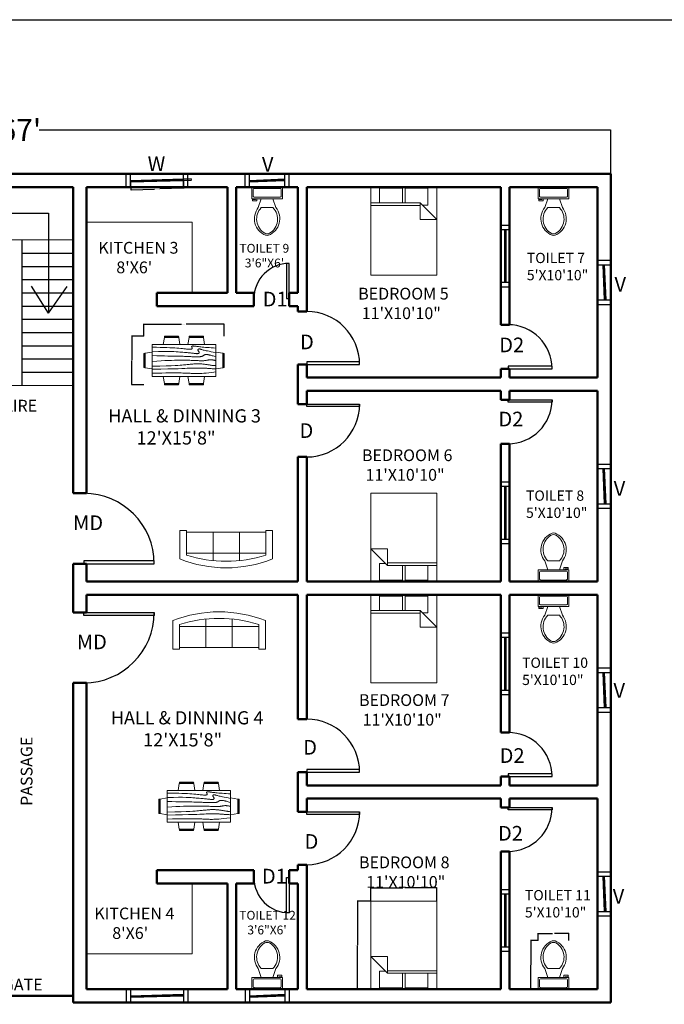
# Model space of a CAD drawing. Units: inches. Extents: x 9239 to 26065, y 6728 to 14611.
# Tile 3 of 12: x 9801 to 10240, y 7264 to 7934. Entities that reach past the tile are written whole.
import ezdxf

# ---------------------------------------------------------------- set-up
doc = ezdxf.new("R2010")
doc.units = ezdxf.units.IN
doc.header["$MEASUREMENT"] = 0
for name, color, linetype, lineweight in [('A-ANNO-DIMS', 2, 'Continuous', 18), ('A-ANNO-TEXT', 7, 'Continuous', 18), ('A-AREA-IDEN', 7, 'Continuous', 18), ('A-DOOR', 4, 'Continuous', 25), ('A-FLOR-FIXT', 8, 'Continuous', 18), ('A-FLOR-STRS', 3, 'Continuous', 25), ('A-FURN', 8, 'Continuous', 18), ('A-GLAZ', 4, 'Continuous', 25), ('A-WALL', 7, 'Continuous', 50)]:
    doc.layers.add(name, color=color, linetype=linetype, lineweight=lineweight)
doc.styles.get("Standard").update_dxf_attribs({"font": 'arial.ttf'})
doc.dimstyles.get("Standard").update_dxf_attribs({"dimtxt": 0.18, "dimasz": 0.18, "dimexe": 0.18, "dimexo": 0.0625, "dimgap": 0.09, "dimtad": 0, "dimtih": 1, "dimtoh": 1, "dimdec": 0, "dimzin": 0, "dimdsep": 46, "dimlunit": 3, "dimtxsty": 'Standard', "dimcen": 0.09, "dimadec": 0, "dimazin": 0, "dimtfac": 1, "dimtdec": 0, "dimtofl": 0, "dimtmove": 0, "dimatfit": 3, "dimfxl": 1, "dimtolj": 1, "dimtzin": 0, "dimarcsym": 0})

# ---------------------------------------------------------------- blocks, each defined once
blk = doc.blocks.new('*U4')
for p, q in [((-24, 0), (-24, 5)), ((0, 0), (0, 5))]:
    blk.add_line(p, q)
blk.add_lwpolyline([(0, 0), (0, -24), (-1.75, -24), (-1.75, 0)], close=True)
blk.add_arc((0, 0), 24, 180, 270)
blk = doc.blocks.new('*U3')
for p, q in [((-24, 0), (-24, -5)), ((0, 0), (0, -5))]:
    blk.add_line(p, q)
blk.add_lwpolyline([(0, 0), (0, 24), (-1.75, 24), (-1.75, 0)], close=True)
blk.add_arc((0, 0), 24, 90, 180)
blk = doc.blocks.new('*U2')
for p, q in [((0, 0), (0, -5)), ((30, 0), (30, -5))]:
    blk.add_line(p, q)
blk.add_lwpolyline([(0, 0), (0, 30), (1.75, 30), (1.75, 0)], close=True)
blk.add_arc((0, 0), 30, 0, 90)
blk = doc.blocks.new('*U7')
for p, q in [((-30, 0), (-30, -5)), ((0, 0), (0, -5))]:
    blk.add_line(p, q)
blk.add_lwpolyline([(0, 0), (0, 30), (-1.75, 30), (-1.75, 0)], close=True)
blk.add_arc((0, 0), 30, 90, 180)
blk = doc.blocks.new('*U10')
for p, q in [((0, 0), (0, -6)), ((36, 0), (36, -6))]:
    blk.add_line(p, q)
blk.add_lwpolyline([(0, 0), (0, 36), (1.75, 36), (1.75, 0)], close=True)
blk.add_arc((0, 0), 36, 0, 90)
blk = doc.blocks.new('*U11')
for p, q in [((0, 0), (0, -6)), ((-36, 0), (-36, -6))]:
    blk.add_line(p, q)
blk.add_lwpolyline([(0, 0), (0, 36), (-1.75, 36), (-1.75, 0)], close=True)
blk.add_arc((0, 0), 36, 90, 180)
blk = doc.blocks.new('*U17')
for p, q in [((0, 0), (0, -6)), ((40, 0), (40, -6))]:
    blk.add_line(p, q)
blk.add_lwpolyline([(0, 0), (0, 40), (1.75, 40), (1.75, 0)], close=True)
blk.add_arc((0, 0), 40, 0, 90)
blk = doc.blocks.new('*U16')
for p, q in [((0, 0), (0, -6)), ((-40, 0), (-40, -6))]:
    blk.add_line(p, q)
blk.add_lwpolyline([(0, 0), (0, 40), (-1.75, 40), (-1.75, 0)], close=True)
blk.add_arc((0, 0), 40, 90, 180)
blk = doc.blocks.new('Bed - Queen')
for p, q in [((0, -80.00003), (0, 0)), ((0, 0), (59.99999, 0)), ((59.99999, 0), (59.99999, -80.00003)), ((7.99999, -1.2), (28.79998, -1.2)), ((7.99999, -14.4), (7.99999, -1.2)), ((28.79998, -1.2), (28.79998, -14.4)), ((31.19999, -1.2), (51.99999, -1.2)), ((31.19999, -14.4), (31.19999, -1.2)), ((51.99999, -1.2), (51.99999, -16.4)), ((0, -14.4), (44.8, -14.4)), ((44.8, -16.8), (0, -16.8)), ((59.99999, -29.6), (44.8, -14.4)), ((44.8, -14.4), (44.8, -29.6)), ((51.99999, -16.4), (46.79936, -16.4)), ((44.8, -29.6), (59.99999, -29.6)), ((59.99999, -80.00003), (0, -80.00003))]:
    blk.add_line(p, q)
blk = doc.blocks.new('Toilet - top')
for p, q in [((9.5, -6), (9.5, -2)), ((-10, -8.5), (-8, -8.5)), ((-10, -9.5), (-10, -8.5)), ((-7, -9.5), (-10, -9.5)), ((-8, -8.5), (-8, -8)), ((-7, -8), (-7, -9.5)), ((-4, -8), (-6, -14)), ((4, -8), (6, -14)), ((4, -14), (-4, -14))]:
    blk.add_line(p, q)
blk.add_lwpolyline([(10.5, -8), (10.5, 0), (-10.5, 0), (-10.5, -8)], close=True)
for points in [[(-9.5, -2), (-9.5, -6)], [(8.5, -1), (-8.5, -1)], [(-8.5, -7), (8.5, -7)]]:
    blk.add_lwpolyline(points)
for centre, radius, start, end in [((-8.62, -1.88), 0.884, 81.8699, 188.1301), ((-8.62, -6.12), 0.884, 171.8699, 278.1301), ((8.62, -1.88), 0.884, 351.8699, 98.1301), ((8.62, -6.12), 0.884, 261.8699, 8.1301), ((3.52, -21.58), 12.17, 141.46911, 247.97143), ((4.2, -21.82), 11.33, 136.36773, 238.94682), ((-3.52, -21.58), 12.17, 292.02843, 38.53071), ((-4.2, -21.82), 11.33, 301.05301, 43.63209), ((0, -27.88), 4, 245.73182, 294.26817), ((0, -29), 4, 254.86053, 285.13947)]:
    blk.add_arc(centre, radius, start, end)
blk = doc.blocks.new('Sofa - Roundback 7 ft.')
for p, q in [((-12.00002, -32.4421), (-12.00003, -6.5971)), ((11.99997, -32.4421), (11.99998, -6.5971)), ((-36.000027, -34), (-36.000027, -11.4696)), ((-35.999844, -13.3819), (35.9998, -13.3819)), ((35.99998, -34), (35.99998, -11.4696)), ((-36.000027, -32.4421), (35.99998, -32.4421))]:
    blk.add_line(p, q)
for points in [[(-36.000027, -34), (-42.000027, -34), (-42.000027, -8)], [(41.99998, -8), (41.99998, -34), (35.99998, -34)]]:
    blk.add_lwpolyline(points)
for centre, radius, start, end in [((0, -114.25), 114.25, 68.43141, 111.5686), ((-0.00001, -127.1968), 121.1968, 72.72033, 107.2797)]:
    blk.add_arc(centre, radius, start, end)
blk = doc.blocks.new('Dining Set - 36 x 72 in.')
for p, q in [((-22.2343, 26.00059), (-23.4847, 17.99762)), ((-22.2304, 26), (-5.7608, 26)), ((-22, 27.5), (-22.1562, 26.50042)), ((-5.8416, 26.5), (-22.1534, 26.5)), ((-22, 27.5), (-6, 27.5)), ((-5.8437, 26.49966), (-6, 27.5)), ((-4.5152, 17.99762), (-5.7655, 25.99926)), ((5.7657, 26.00059), (4.5153, 17.99762)), ((5.7696, 26), (22.2392, 26)), ((6, 27.5), (5.8438, 26.50042)), ((22.1584, 26.5), (5.8466, 26.5)), ((6, 27.5), (22, 27.5)), ((22.1563, 26.49966), (22, 27.5)), ((23.4848, 17.99762), (22.2345, 25.99926)), ((36, 18), (-36, 18)), ((-36, 18), (-36, -18)), ((36, -18), (36, 18)), ((-45.5, 8), (-44.5004, 8.15617)), ((-45.5, 8), (-45.5, -8)), ((-44.5, -8.15843), (-44.5, 8.15338)), ((-44.0006, 8.23428), (-35.9976, 9.48474)), ((-44, 8.23041), (-44, -8.23915)), ((44.0006, 8.23428), (35.9976, 9.48474)), ((44, 8.23041), (44, -8.23915)), ((44.5, -8.15843), (44.5, 8.15338)), ((45.5, 8), (44.5005, 8.15617)), ((45.5, 8), (45.5, -8)), ((-44.4997, -8.15631), (-45.5, -8)), ((-35.9976, -9.48476), (-43.9993, -8.2345)), ((35.9976, -9.48476), (43.9993, -8.2345)), ((44.4997, -8.15631), (45.5, -8)), ((-36, -18), (36, -18)), ((-22.2343, -26.0006), (-23.4847, -17.99762)), ((-4.5152, -17.99762), (-5.7655, -25.99928)), ((5.7657, -26.0006), (4.5153, -17.99762)), ((23.4848, -17.99762), (22.2345, -25.99928)), ((-22.2304, -26), (-5.7608, -26)), ((-22, -27.5), (-22.1562, -26.50044)), ((-5.8416, -26.5), (-22.1534, -26.5)), ((-22, -27.5), (-6, -27.5)), ((-5.8437, -26.49967), (-6, -27.5)), ((5.7696, -26), (22.2392, -26)), ((6, -27.5), (5.8438, -26.50044)), ((22.1584, -26.5), (5.8466, -26.5)), ((6, -27.5), (22, -27.5)), ((22.1563, -26.49967), (22, -27.5))]:
    blk.add_line(p, q)
for points in [[(-36, 15), (-31.1772, 14.97754), (-26.8079, 14.91406), (-22.8538, 14.81543), (-19.276, 14.6875), (-16.0362, 14.53613), (-13.0957, 14.36718), (-10.4159, 14.18652), (-7.9583, 14), (-5.6904, 13.81315), (-3.6035, 13.63021), (-1.6954, 13.45508), (0.0365, 13.29166), (1.5945, 13.14388), (2.9811, 13.01562), (4.1988, 12.9108), (5.25, 12.83333), (6.1393, 12.78613), (6.8802, 12.76823), (7.4883, 12.77767), (7.9792, 12.8125), (8.3685, 12.87077), (8.6719, 12.95052), (8.9049, 13.0498), (9.0833, 13.16666), (9.2205, 13.29899), (9.3216, 13.44401), (9.3895, 13.59879), (9.4271, 13.76041), (9.4373, 13.92594), (9.4232, 14.09245), (9.3875, 14.257), (9.3333, 14.41666), (9.2638, 14.56917), (9.1836, 14.71484), (9.0975, 14.85465), (9.0104, 14.98958), (8.9272, 15.1206), (8.8529, 15.2487), (8.7922, 15.37483), (8.75, 15.5), (8.7305, 15.62467), (8.7344, 15.74739), (8.7617, 15.86621), (8.8125, 15.97916), (8.8867, 16.08431), (8.9844, 16.17968), (9.1055, 16.26334), (9.25, 16.33333), (9.4189, 16.38802), (9.6172, 16.42708), (9.8506, 16.45052), (10.125, 16.45833), (10.4463, 16.45052), (10.8203, 16.42708), (11.2529, 16.38802), (11.75, 16.33333), (12.3184, 16.26318), (12.9694, 16.17838), (13.7151, 16.07991), (14.5677, 15.96875), (15.5395, 15.84586), (16.6426, 15.71224), (17.8893, 15.56884), (19.2917, 15.41666), (20.859, 15.25667), (22.5879, 15.08984), (24.4721, 14.91715), (26.5052, 14.73958), (28.6809, 14.5581), (30.9929, 14.3737), (33.4347, 14.18733), (36, 14)], [(-36, 10), (-28.9766, 10.14274), (-23.1725, 10.20442), (-18.4241, 10.19775), (-14.5677, 10.13541), (-11.4399, 10.03011), (-8.877, 9.89453), (-6.7154, 9.74137), (-4.7917, 9.58333), (-2.9698, 9.43082), (-1.2246, 9.28515), (0.4415, 9.14534), (2.026, 9.01041), (3.5266, 8.87939), (4.9408, 8.7513), (6.266, 8.62516), (7.5, 8.5), (8.6411, 8.37549), (9.6914, 8.2539), (10.6538, 8.13818), (11.5312, 8.03125), (12.3267, 7.93603), (13.043, 7.85547), (13.6831, 7.79248), (14.25, 7.75), (14.7471, 7.7303), (15.1797, 7.73307), (15.5537, 7.75732), (15.875, 7.80208), (16.1494, 7.86637), (16.3828, 7.94922), (16.5811, 8.04964), (16.75, 8.16666), (16.8944, 8.29915), (17.0143, 8.44531), (17.1089, 8.60319), (17.1771, 8.77083), (17.218, 8.94629), (17.2305, 9.1276), (17.2137, 9.31282), (17.1667, 9.5), (17.0895, 9.6875), (16.987, 9.875), (16.8649, 10.0625), (16.7292, 10.25), (16.5856, 10.4375), (16.4401, 10.625), (16.2985, 10.8125), (16.1667, 11), (16.05, 11.18733), (15.9518, 11.3737), (15.8752, 11.5581), (15.8229, 11.73958), (15.798, 11.91715), (15.8034, 12.08984), (15.842, 12.25667), (15.9167, 12.41666), (16.0295, 12.56836), (16.1784, 12.70833), (16.3605, 12.83268), (16.5729, 12.9375), (16.8127, 13.01888), (17.0768, 13.07291), (17.3625, 13.0957), (17.6667, 13.08333), (17.9894, 13.03312), (18.3418, 12.94726), (18.7382, 12.82918), (19.1927, 12.68229), (19.7195, 12.51001), (20.3327, 12.31575), (21.0465, 12.10294), (21.875, 11.875), (22.8357, 11.63354), (23.959, 11.37304), (25.2786, 11.08618), (26.8282, 10.76562), (28.6414, 10.40405), (30.752, 9.99414), (33.1936, 9.52856), (36, 9)], [(-36, 5.5), (-30.7157, 5.3348), (-26.069, 5.20963), (-21.9946, 5.11767), (-18.4271, 5.05208), (-15.3009, 5.00602), (-12.5508, 4.97265), (-10.1112, 4.94515), (-7.9167, 4.91666), (-5.909, 4.88167), (-4.0586, 4.83984), (-2.3429, 4.79215), (-0.7396, 4.73958), (0.7739, 4.6831), (2.22, 4.6237), (3.6213, 4.56233), (5, 4.5), (6.373, 4.43782), (7.7344, 4.3776), (9.0723, 4.32129), (10.375, 4.27083), (11.6309, 4.22819), (12.8281, 4.19531), (13.9551, 4.17415), (15, 4.16666), (15.954, 4.17448), (16.819, 4.19791), (17.6001, 4.23698), (18.3021, 4.29166), (18.9299, 4.36198), (19.4883, 4.44791), (19.9823, 4.54948), (20.4167, 4.66666), (20.7969, 4.79899), (21.1302, 4.94401), (21.4245, 5.09879), (21.6875, 5.26041), (21.9271, 5.42594), (22.1511, 5.59245), (22.3672, 5.757), (22.5834, 5.91666), (22.8065, 6.06868), (23.0404, 6.21093), (23.2879, 6.34147), (23.5521, 6.45833), (23.8358, 6.55957), (24.142, 6.64323), (24.4735, 6.70735), (24.8334, 6.75), (25.2235, 6.76969), (25.642, 6.76692), (26.0858, 6.74267), (26.5521, 6.69791), (27.0379, 6.63362), (27.5404, 6.55078), (28.0565, 6.45036), (28.5834, 6.33333), (29.1242, 6.19987), (29.7071, 6.04687), (30.3661, 5.87044), (31.1354, 5.66666), (32.0493, 5.43164), (33.142, 5.16146), (34.4475, 4.85221), (36, 4.5)], [(-36, -1), (-30.7915, -0.6591), (-26.0195, -0.38216), (-21.6519, -0.16284), (-17.6563, 0.00521), (-14.0005, 0.12833), (-10.6523, 0.21289), (-7.5796, 0.26522), (-4.75, 0.29166), (-2.134, 0.29793), (0.2878, 0.28711), (2.5317, 0.26163), (4.6146, 0.22396), (6.5529, 0.17651), (8.3633, 0.12174), (10.0623, 0.06209), (11.6667, 0), (13.1899, -0.06201), (14.6341, -0.1211), (15.9982, -0.17432), (17.2813, -0.21875), (18.4823, -0.25147), (19.6003, -0.26953), (20.6343, -0.27002), (21.5834, -0.25), (22.4481, -0.20768), (23.2357, -0.14584), (23.9549, -0.06836), (24.6146, 0.02083), (25.2235, 0.11784), (25.7904, 0.21875), (26.3241, 0.31966), (26.8334, 0.41666), (27.3265, 0.50618), (27.8099, 0.58593), (28.2894, 0.65397), (28.7709, 0.70833), (29.2601, 0.74707), (29.763, 0.76823), (30.2855, 0.76985), (30.8334, 0.75), (31.4088, 0.70784), (31.9994, 0.64713), (32.589, 0.57275), (33.1615, 0.48958), (33.7008, 0.4025), (34.1908, 0.3164), (34.6153, 0.23616), (34.9584, 0.16666), (35.2099, 0.11165), (35.3848, 0.07031), (35.504, 0.04069), (35.5886, 0.02083), (35.6594, 0.00879), (35.7377, 0.0026), (35.8442, 0.00032), (36, 0)], [(-36, -6.5), (-27.1843, -6.31267), (-20.084, -6.1263), (-14.469, -5.9419), (-10.1094, -5.76042), (-6.7752, -5.58285), (-4.2363, -5.41016), (-2.2629, -5.24333), (-0.625, -5.08334), (0.8708, -4.93099), (2.2715, -4.78646), (3.5872, -4.64974), (4.8281, -4.52084), (6.0046, -4.39974), (7.127, -4.28646), (8.2053, -4.18099), (9.25, -4.08334), (10.2705, -3.99382), (11.2734, -3.91407), (12.2647, -3.84603), (13.25, -3.79167), (14.2354, -3.75293), (15.2266, -3.73177), (16.2295, -3.73015), (17.25, -3.75), (18.2912, -3.79248), (19.3451, -3.85547), (20.4009, -3.93604), (21.4479, -4.03125), (22.4754, -4.13819), (23.4727, -4.25391), (24.4289, -4.37549), (25.3334, -4.5), (26.1785, -4.62492), (26.9694, -4.74935), (27.7145, -4.87281), (28.4219, -4.99479), (29.1, -5.11483), (29.7572, -5.23242), (30.4016, -5.34709), (31.0417, -5.45834), (31.6837, -5.56437), (32.3262, -5.65821), (32.9658, -5.73153), (33.599, -5.77604), (34.2224, -5.78345), (34.8327, -5.74545), (35.4264, -5.65373), (36, -5.5)], [(-36, -10), (-26.4022, -9.81299), (-18.4675, -9.62891), (-11.9839, -9.45069), (-6.7396, -9.28125), (-2.5226, -9.12354), (0.8789, -8.98047), (3.6769, -8.85498), (6.0833, -8.75), (8.2767, -8.66765), (10.3021, -8.60677), (12.1712, -8.56543), (13.8958, -8.54167), (15.4876, -8.53353), (16.9583, -8.53907), (18.3197, -8.55632), (19.5834, -8.58334), (20.7616, -8.61841), (21.8685, -8.66081), (22.9188, -8.71004), (23.9271, -8.76563), (24.9081, -8.82707), (25.8763, -8.89388), (26.8465, -8.96558), (27.8334, -9.04167), (28.8474, -9.12118), (29.8828, -9.20117), (30.93, -9.27824), (31.9792, -9.34896), (33.0205, -9.40991), (34.0443, -9.45768), (35.0407, -9.48885), (36, -9.5)], [(-36, -14.5), (-30.0881, -14.33513), (-25.0332, -14.21224), (-20.7312, -14.12647), (-17.0781, -14.07292), (-13.97, -14.04671), (-11.3027, -14.04297), (-8.9724, -14.05681), (-6.875, -14.08334), (-4.9224, -14.11833), (-3.0905, -14.16016), (-1.3709, -14.20785), (0.2448, -14.26042), (1.7647, -14.3169), (3.1973, -14.3763), (4.5507, -14.43767), (5.8333, -14.5), (7.0554, -14.5621), (8.235, -14.62175), (9.3922, -14.67652), (10.5469, -14.72396), (11.7192, -14.76164), (12.929, -14.78711), (14.1965, -14.79794), (15.5417, -14.79167), (16.9933, -14.76424), (18.6152, -14.70508), (20.4804, -14.60197), (22.6615, -14.44271), (25.2312, -14.21509), (28.2624, -13.9069), (31.8277, -13.50594), (36, -13)]]:
    blk.add_lwpolyline(points)
blk = doc.blocks.new('*D22')
at = {"layer": 'A-ANNO-DIMS', "color": 0, "lineweight": -2, "transparency": 16777216}
for p, q in [((9399.35, 7829.13), (9399.35, 7858.98)), ((9399.53, 7858.8), (9788.49, 7858.8)), ((10203.17, 7858.8), (9814.21, 7858.8)), ((10203.35, 7829.13), (10203.35, 7858.98))]:
    blk.add_line(p, q, dxfattribs=at)
at = {"layer": 'A-ANNO-DIMS', "color": 0, "transparency": 16777216}
for points in [[(9399.53, 7858.83), (9399.53, 7858.77), (9399.35, 7858.8)], [(10203.17, 7858.83), (10203.17, 7858.77), (10203.35, 7858.8)]]:
    blk.add_solid(points, dxfattribs=at)
at = {"layer": 'Defpoints', "color": 0, "transparency": 16777216}
for p in [(10203.35, 7858.8), (9399.35, 7829.07), (10203.35, 7829.07)]:
    blk.add_point(p, dxfattribs=at)
at = {"layer": 'A-ANNO-DIMS', "color": 0, "transparency": 16777216, "insert": (9801.35, 7858.8), "char_height": 0.18, "attachment_point": 5}
blk.add_mtext("\\A1;{\\H83.33333x;67'}", dxfattribs=at)
blk = doc.blocks.new('WIN-36')
for p, q in [((0, 1), (36, 1)), ((0, 0.5), (36, 0.5)), ((0, 0), (36, 0))]:
    blk.add_line(p, q)
blk = doc.blocks.new('WIN-24')
for p, q in [((0, 1), (24, 1)), ((0, 0.5), (24, 0.5)), ((0, 0), (24, 0))]:
    blk.add_line(p, q)
blk = doc.blocks.new('*D40')
at = {"layer": 'A-ANNO-DIMS', "color": 0, "lineweight": -2, "transparency": 16777216}
for p, q in [((9876.37, 7823.51), (9876.53, 7817.99)), ((9912.36, 7824.51), (9912.51, 7818.99)), ((9876.7, 7818.18), (9892.76, 7818.62)), ((9912.33, 7819.17), (9896.27, 7818.72))]:
    blk.add_line(p, q, dxfattribs=at)
at = {"layer": 'A-ANNO-DIMS', "color": 0, "transparency": 16777216}
for points in [[(9876.7, 7818.21), (9876.7, 7818.15), (9876.52, 7818.17)], [(9912.33, 7819.2), (9912.33, 7819.14), (9912.51, 7819.17)]]:
    blk.add_solid(points, dxfattribs=at)
at = {"layer": 'Defpoints', "color": 0, "transparency": 16777216}
for p in [(9876.37, 7823.57), (9912.36, 7824.57), (9912.51, 7819.17)]:
    blk.add_point(p, dxfattribs=at)
at = {"layer": 'A-ANNO-DIMS', "color": 0, "transparency": 16777216, "insert": (9894.52, 7818.67), "char_height": 0.18, "attachment_point": 5}
blk.add_mtext('\\A1;WINDOW W (3\'-0") 3\'-0" TYP.', dxfattribs=at)
blk = doc.blocks.new('*D41')
at = {"layer": 'A-ANNO-DIMS', "color": 0, "lineweight": -2, "transparency": 16777216}
for p, q in [((9912.39, 7825.57), (9917.91, 7825.73)), ((9912.42, 7824.57), (9917.94, 7824.73)), ((9917.73, 7825.54), (9917.74, 7825.4)), ((9917.75, 7824.9), (9917.75, 7825.04))]:
    blk.add_line(p, q, dxfattribs=at)
at = {"layer": 'A-ANNO-DIMS', "color": 0, "transparency": 16777216}
for points in [[(9917.76, 7825.54), (9917.7, 7825.54), (9917.73, 7825.72)], [(9917.78, 7824.9), (9917.72, 7824.9), (9917.76, 7824.72)]]:
    blk.add_solid(points, dxfattribs=at)
at = {"layer": 'Defpoints', "color": 0, "transparency": 16777216}
for p in [(9912.33, 7825.57), (9912.36, 7824.57), (9917.73, 7825.72)]:
    blk.add_point(p, dxfattribs=at)
at = {"layer": 'A-ANNO-DIMS', "color": 0, "transparency": 16777216, "insert": (9917.74, 7825.22), "char_height": 0.18, "attachment_point": 5}
blk.add_mtext('\\A1;0\'-1" TYP.', dxfattribs=at)
blk = doc.blocks.new('*D44')
at = {"layer": 'A-ANNO-DIMS', "color": 0, "lineweight": -2, "transparency": 16777216}
for p, q in [((10039.79, 7334.07), (10030.67, 7334.07)), ((10030.85, 7333.89), (10030.85, 7304.26)), ((10030.85, 7274.25), (10030.85, 7303.88)), ((10039.79, 7274.07), (10030.67, 7274.07))]:
    blk.add_line(p, q, dxfattribs=at)
at = {"layer": 'A-ANNO-DIMS', "color": 0, "transparency": 16777216}
for points in [[(10030.82, 7333.89), (10030.88, 7333.89), (10030.85, 7334.07)], [(10030.82, 7274.25), (10030.88, 7274.25), (10030.85, 7274.07)]]:
    blk.add_solid(points, dxfattribs=at)
at = {"layer": 'Defpoints', "color": 0, "transparency": 16777216}
for p in [(10039.85, 7334.07), (10030.85, 7274.07), (10039.85, 7274.07)]:
    blk.add_point(p, dxfattribs=at)
at = {"layer": 'A-ANNO-DIMS', "color": 0, "transparency": 16777216, "insert": (10030.85, 7304.07), "char_height": 0.18, "attachment_point": 5}
blk.add_mtext('\\A1;QUEEN BED 5\'-0" TYP.', dxfattribs=at)
blk = doc.blocks.new('*D45')
at = {"layer": 'A-ANNO-DIMS', "color": 0, "lineweight": -2, "transparency": 16777216}
for p, q in [((10039.85, 7334.13), (10039.85, 7343.25)), ((10040.03, 7343.07), (10061.71, 7343.07)), ((10084.67, 7343.07), (10062.99, 7343.07)), ((10084.85, 7334.13), (10084.85, 7343.25))]:
    blk.add_line(p, q, dxfattribs=at)
at = {"layer": 'A-ANNO-DIMS', "color": 0, "transparency": 16777216}
for points in [[(10040.03, 7343.1), (10040.03, 7343.04), (10039.85, 7343.07)], [(10084.67, 7343.1), (10084.67, 7343.04), (10084.85, 7343.07)]]:
    blk.add_solid(points, dxfattribs=at)
at = {"layer": 'Defpoints', "color": 0, "transparency": 16777216}
for p in [(10039.85, 7343.07), (10039.85, 7334.07), (10084.85, 7334.07)]:
    blk.add_point(p, dxfattribs=at)
at = {"layer": 'A-ANNO-DIMS', "color": 0, "transparency": 16777216, "insert": (10062.35, 7343.07), "char_height": 0.18, "attachment_point": 5}
blk.add_mtext('\\A1;3\'-9" TYP.', dxfattribs=at)
blk = doc.blocks.new('*D50')
at = {"layer": 'A-ANNO-DIMS', "color": 0, "lineweight": -2, "transparency": 16777216}
for p, q in [((10153.79, 7307.12), (10148.71, 7307.12)), ((10148.89, 7306.94), (10148.89, 7290.78)), ((10148.89, 7274.25), (10148.89, 7290.41)), ((10153.79, 7274.07), (10148.71, 7274.07))]:
    blk.add_line(p, q, dxfattribs=at)
at = {"layer": 'A-ANNO-DIMS', "color": 0, "transparency": 16777216}
for points in [[(10148.86, 7306.94), (10148.92, 7306.94), (10148.89, 7307.12)], [(10148.86, 7274.25), (10148.92, 7274.25), (10148.89, 7274.07)]]:
    blk.add_solid(points, dxfattribs=at)
at = {"layer": 'Defpoints', "color": 0, "transparency": 16777216}
for p in [(10153.85, 7307.12), (10148.89, 7274.07), (10153.85, 7274.07)]:
    blk.add_point(p, dxfattribs=at)
at = {"layer": 'A-ANNO-DIMS', "color": 0, "transparency": 16777216, "insert": (10148.89, 7290.59), "char_height": 0.18, "attachment_point": 5}
blk.add_mtext('\\A1;WC 2\'-9" TYP.', dxfattribs=at)
blk = doc.blocks.new('*D51')
at = {"layer": 'A-ANNO-DIMS', "color": 0, "lineweight": -2, "transparency": 16777216}
for p, q in [((10153.85, 7307.18), (10153.85, 7312.25)), ((10154.03, 7312.07), (10163.72, 7312.07)), ((10174.67, 7312.07), (10164.98, 7312.07)), ((10174.85, 7307.18), (10174.85, 7312.25))]:
    blk.add_line(p, q, dxfattribs=at)
at = {"layer": 'A-ANNO-DIMS', "color": 0, "transparency": 16777216}
for points in [[(10154.03, 7312.1), (10154.03, 7312.04), (10153.85, 7312.07)], [(10174.67, 7312.1), (10174.67, 7312.04), (10174.85, 7312.07)]]:
    blk.add_solid(points, dxfattribs=at)
at = {"layer": 'Defpoints', "color": 0, "transparency": 16777216}
for p in [(10153.85, 7312.07), (10153.85, 7307.12), (10174.85, 7307.12)]:
    blk.add_point(p, dxfattribs=at)
at = {"layer": 'A-ANNO-DIMS', "color": 0, "transparency": 16777216, "insert": (10164.35, 7312.07), "char_height": 0.18, "attachment_point": 5}
blk.add_mtext('\\A1;1\'-9" TYP.', dxfattribs=at)
blk = doc.blocks.new('*D56')
at = {"layer": 'A-ANNO-DIMS', "color": 0, "lineweight": -2, "transparency": 16777216}
for p, q in [((9885.43, 7718.55), (9885.43, 7726.86)), ((9885.61, 7726.68), (9911.13, 7726.68)), ((9939.85, 7726.68), (9914.33, 7726.68)), ((9940.03, 7718.55), (9940.03, 7726.86))]:
    blk.add_line(p, q, dxfattribs=at)
at = {"layer": 'A-ANNO-DIMS', "color": 0, "transparency": 16777216}
for points in [[(9885.61, 7726.71), (9885.61, 7726.65), (9885.43, 7726.68)], [(9939.85, 7726.71), (9939.85, 7726.65), (9940.03, 7726.68)]]:
    blk.add_solid(points, dxfattribs=at)
at = {"layer": 'Defpoints', "color": 0, "transparency": 16777216}
for p in [(9940.03, 7726.68), (9885.43, 7718.49), (9940.03, 7718.49)]:
    blk.add_point(p, dxfattribs=at)
at = {"layer": 'A-ANNO-DIMS', "color": 0, "transparency": 16777216, "insert": (9912.73, 7726.68), "char_height": 0.18, "attachment_point": 5}
blk.add_mtext('\\A1;DINING SET 4\'-6 1/2" TYP.', dxfattribs=at)
blk = doc.blocks.new('*D57')
at = {"layer": 'A-ANNO-DIMS', "color": 0, "lineweight": -2, "transparency": 16777216}
for p, q in [((9885.37, 7718.49), (9877.06, 7718.49)), ((9877.24, 7718.31), (9877.24, 7702.17)), ((9877.24, 7685.67), (9877.24, 7701.81)), ((9885.37, 7685.49), (9877.06, 7685.49))]:
    blk.add_line(p, q, dxfattribs=at)
at = {"layer": 'A-ANNO-DIMS', "color": 0, "transparency": 16777216}
for points in [[(9877.21, 7718.31), (9877.27, 7718.31), (9877.24, 7718.49)], [(9877.21, 7685.67), (9877.27, 7685.67), (9877.24, 7685.49)]]:
    blk.add_solid(points, dxfattribs=at)
at = {"layer": 'Defpoints', "color": 0, "transparency": 16777216}
for p in [(9877.24, 7718.49), (9885.43, 7718.49), (9885.43, 7685.49)]:
    blk.add_point(p, dxfattribs=at)
at = {"layer": 'A-ANNO-DIMS', "color": 0, "transparency": 16777216, "insert": (9877.24, 7701.99), "char_height": 0.18, "attachment_point": 5}
blk.add_mtext('\\A1;2\'-9" TYP.', dxfattribs=at)

msp = doc.modelspace()

# ---------------------------------------------------------------- linework, layer by layer
at = {"layer": 'A-FLOR-FIXT'}
for p, q in [((9846.35, 7796.07), (9918.35, 7796.07)), ((9918.35, 7796.07), (9918.35, 7748.07)), ((9765.35, 7784.07), (9837.35, 7784.07)), ((9765.35, 7685.07), (9837.35, 7685.07)), ((9918.35, 7346.07), (9918.35, 7298.07)), ((9918.35, 7298.07), (9846.35, 7298.07))]:
    msp.add_line(p, q, dxfattribs=at)
at = {"layer": 'A-FLOR-STRS'}
for p, q in [((9783.59, 7802.23), (9820.58, 7802.23)), ((9820.58, 7802.23), (9820.58, 7734.26)), ((9802.35, 7784.07), (9802.35, 7685.07)), ((9802.35, 7775.07), (9837.35, 7775.07)), ((9802.35, 7766.07), (9837.35, 7766.07)), ((9802.35, 7757.07), (9837.35, 7757.07)), ((9802.35, 7748.07), (9837.35, 7748.07)), ((9820.58, 7734.26), (9808.9, 7752.55)), ((9820.58, 7734.26), (9833.25, 7752.45)), ((9802.35, 7739.07), (9837.35, 7739.07)), ((9802.35, 7730.07), (9837.35, 7730.07)), ((9802.35, 7721.07), (9837.35, 7721.07)), ((9802.35, 7712.07), (9837.35, 7712.07)), ((9802.35, 7703.07), (9837.35, 7703.07)), ((9802.35, 7694.07), (9837.35, 7694.07))]:
    msp.add_line(p, q, dxfattribs=at)
msp.add_lwpolyline([(9238.6, 7933.95), (11208.24, 7933.95), (11208.24, 6728.19), (9238.6, 6728.19)], close=True, dxfattribs=at)
at = {"layer": 'A-GLAZ'}
for p, q in [((9873.35, 7820.07), (9873.35, 7829.07)), ((9876.35, 7820.07), (9876.35, 7829.07)), ((9912.35, 7820.07), (9912.35, 7829.07)), ((9915.35, 7820.07), (9915.35, 7829.07)), ((9954.35, 7820.07), (9954.35, 7829.07)), ((9957.35, 7820.07), (9957.35, 7829.07)), ((9981.35, 7820.07), (9981.35, 7829.07)), ((9984.35, 7820.07), (9984.35, 7829.07)), ((10128.35, 7794.2), (10134.35, 7794.2)), ((10128.35, 7791.2), (10134.35, 7791.2)), ((10130.85, 7791.2), (10130.85, 7755.2)), ((10131.35, 7791.2), (10131.35, 7755.2)), ((10131.85, 7791.2), (10131.85, 7755.2)), ((10194.35, 7770.2), (10203.35, 7770.2)), ((10194.35, 7767.2), (10203.35, 7767.2)), ((10128.35, 7755.2), (10134.35, 7755.2)), ((10128.35, 7752.2), (10134.35, 7752.2)), ((10194.35, 7743.2), (10203.35, 7743.2)), ((10194.35, 7740.2), (10203.35, 7740.2)), ((10194.35, 7631.45), (10203.35, 7631.45)), ((10194.35, 7628.45), (10203.35, 7628.45)), ((10128.35, 7619.45), (10134.35, 7619.45)), ((10128.35, 7616.45), (10134.35, 7616.45)), ((10130.85, 7616.45), (10130.85, 7580.45)), ((10131.35, 7616.45), (10131.35, 7580.45)), ((10131.85, 7616.45), (10131.85, 7580.45)), ((10194.35, 7604.45), (10203.35, 7604.45)), ((10194.35, 7601.45), (10203.35, 7601.45)), ((10128.35, 7580.45), (10134.35, 7580.45)), ((10128.35, 7577.45), (10134.35, 7577.45)), ((10128.35, 7516.7), (10134.35, 7516.7)), ((10128.35, 7513.7), (10134.35, 7513.7)), ((10130.85, 7513.7), (10130.85, 7477.7)), ((10131.35, 7513.7), (10131.35, 7477.7)), ((10131.85, 7513.7), (10131.85, 7477.7)), ((10194.35, 7492.7), (10203.35, 7492.7)), ((10194.35, 7489.7), (10203.35, 7489.7)), ((10128.35, 7477.7), (10134.35, 7477.7)), ((10128.35, 7474.7), (10134.35, 7474.7)), ((10194.35, 7465.7), (10203.35, 7465.7)), ((10194.35, 7462.7), (10203.35, 7462.7)), ((10194.35, 7353.95), (10203.35, 7353.95)), ((10194.35, 7350.95), (10203.35, 7350.95)), ((10128.35, 7341.95), (10134.35, 7341.95)), ((10128.35, 7338.95), (10134.35, 7338.95)), ((10130.85, 7338.95), (10130.85, 7302.95)), ((10131.35, 7338.95), (10131.35, 7302.95)), ((10131.85, 7338.95), (10131.85, 7302.95)), ((10194.35, 7326.95), (10203.35, 7326.95)), ((10194.35, 7323.95), (10203.35, 7323.95)), ((10128.35, 7302.95), (10134.35, 7302.95)), ((10128.35, 7299.95), (10134.35, 7299.95)), ((9873.35, 7274.07), (9873.35, 7265.07)), ((9876.35, 7274.07), (9876.35, 7265.07)), ((9912.35, 7274.07), (9912.35, 7265.07)), ((9915.35, 7274.07), (9915.35, 7265.07)), ((9954.35, 7274.07), (9954.35, 7265.07)), ((9957.35, 7274.07), (9957.35, 7265.07)), ((9981.35, 7274.07), (9981.35, 7265.07)), ((9984.35, 7274.07), (9984.35, 7265.07))]:
    msp.add_line(p, q, dxfattribs=at)
at = {"layer": 'A-WALL'}
for p, q in [((9399.35, 7829.07), (10203.35, 7829.07)), ((10203.35, 7829.07), (10203.35, 7265.07)), ((9765.35, 7820.07), (9837.35, 7820.07)), ((9837.35, 7820.07), (9837.35, 7611.57)), ((9846.35, 7820.07), (9846.35, 7611.57)), ((9846.35, 7820.07), (9942.35, 7820.07)), ((9942.35, 7820.07), (9942.35, 7748.07)), ((9948.35, 7820.07), (9948.35, 7748.07)), ((9948.35, 7820.07), (9990.35, 7820.07)), ((9990.35, 7820.07), (9990.35, 7748.07)), ((9996.35, 7820.07), (9996.35, 7735.32)), ((9996.35, 7820.07), (10128.35, 7820.07)), ((10128.35, 7820.07), (10128.35, 7726.32)), ((10134.35, 7820.07), (10134.35, 7726.32)), ((10134.35, 7820.07), (10194.35, 7820.07)), ((10194.35, 7820.07), (10194.35, 7690.32)), ((9894.35, 7748.07), (9894.35, 7739.07)), ((9894.35, 7748.07), (9942.35, 7748.07)), ((9948.35, 7748.07), (9960.35, 7748.07)), ((9960.35, 7748.07), (9960.35, 7739.07)), ((9984.35, 7748.07), (9984.35, 7739.07)), ((9984.35, 7748.07), (9990.35, 7748.07)), ((9894.35, 7739.07), (9960.35, 7739.07)), ((9984.35, 7739.07), (9990.35, 7739.07)), ((9990.35, 7739.07), (9990.35, 7735.32)), ((9996.35, 7735.32), (9990.35, 7735.32)), ((10134.35, 7726.32), (10128.35, 7726.32)), ((9996.35, 7699.32), (9990.35, 7699.32)), ((9990.35, 7699.32), (9990.35, 7672.32)), ((9996.35, 7699.32), (9996.35, 7690.32)), ((10134.35, 7696.32), (10128.35, 7696.32)), ((10128.35, 7696.32), (10128.35, 7690.32)), ((10134.35, 7696.32), (10134.35, 7690.32)), ((10128.35, 7690.32), (9996.35, 7690.32)), ((10194.35, 7690.32), (10134.35, 7690.32)), ((9996.35, 7681.32), (9996.35, 7672.32)), ((10128.35, 7681.32), (9996.35, 7681.32)), ((10128.35, 7681.32), (10128.35, 7675.32)), ((10194.35, 7681.32), (10134.35, 7681.32)), ((10134.35, 7681.32), (10134.35, 7675.32)), ((10194.35, 7681.32), (10194.35, 7551.57)), ((10134.35, 7675.32), (10128.35, 7675.32)), ((9996.35, 7672.32), (9990.35, 7672.32)), ((10134.35, 7645.32), (10128.35, 7645.32)), ((10128.35, 7645.32), (10128.35, 7551.57)), ((10134.35, 7645.32), (10134.35, 7551.57)), ((9996.35, 7636.32), (9990.35, 7636.32)), ((9990.35, 7636.32), (9990.35, 7551.57)), ((9996.35, 7636.32), (9996.35, 7551.57)), ((9837.35, 7611.57), (9846.35, 7611.57)), ((9837.35, 7563.57), (9846.35, 7563.57)), ((9837.35, 7563.57), (9837.35, 7530.57)), ((9846.35, 7563.57), (9846.35, 7551.57)), ((9846.35, 7551.57), (9990.35, 7551.57)), ((9996.35, 7551.57), (10128.35, 7551.57)), ((10134.35, 7551.57), (10194.35, 7551.57)), ((9846.35, 7542.57), (9990.35, 7542.57)), ((9846.35, 7542.57), (9846.35, 7530.57)), ((9990.35, 7542.57), (9990.35, 7457.82)), ((9996.35, 7542.57), (9996.35, 7457.82)), ((9996.35, 7542.57), (10128.35, 7542.57)), ((10128.35, 7542.57), (10128.35, 7448.82)), ((10134.35, 7542.57), (10134.35, 7448.82)), ((10134.35, 7542.57), (10194.35, 7542.57)), ((10194.35, 7542.57), (10194.35, 7412.82)), ((9837.35, 7530.57), (9846.35, 7530.57)), ((9837.35, 7482.57), (9846.35, 7482.57)), ((9837.35, 7482.57), (9837.35, 7265.07)), ((9846.35, 7482.57), (9846.35, 7274.07)), ((9996.35, 7457.82), (9990.35, 7457.82)), ((10134.35, 7448.82), (10128.35, 7448.82)), ((9996.35, 7421.82), (9990.35, 7421.82)), ((9990.35, 7421.82), (9990.35, 7394.82)), ((9996.35, 7421.82), (9996.35, 7412.82)), ((10134.35, 7418.82), (10128.35, 7418.82)), ((10128.35, 7418.82), (10128.35, 7412.82)), ((10134.35, 7418.82), (10134.35, 7412.82)), ((10128.35, 7412.82), (9996.35, 7412.82)), ((10194.35, 7412.82), (10134.35, 7412.82)), ((9996.35, 7403.82), (9996.35, 7394.82)), ((10128.35, 7403.82), (9996.35, 7403.82)), ((10128.35, 7403.82), (10128.35, 7397.82)), ((10194.35, 7403.82), (10134.35, 7403.82)), ((10134.35, 7403.82), (10134.35, 7397.82)), ((10194.35, 7403.82), (10194.35, 7274.07)), ((9996.35, 7394.82), (9990.35, 7394.82)), ((10134.35, 7397.82), (10128.35, 7397.82)), ((10134.35, 7367.82), (10128.35, 7367.82)), ((10128.35, 7367.82), (10128.35, 7274.07)), ((10134.35, 7367.82), (10134.35, 7274.07)), ((9996.35, 7358.82), (9990.35, 7358.82)), ((9990.35, 7358.82), (9990.35, 7355.07)), ((9996.35, 7358.82), (9996.35, 7274.07)), ((9894.35, 7355.07), (9894.35, 7346.07)), ((9960.35, 7355.07), (9894.35, 7355.07)), ((9960.35, 7355.07), (9960.35, 7346.07)), ((9990.35, 7355.07), (9984.35, 7355.07)), ((9984.35, 7355.07), (9984.35, 7346.07)), ((9942.35, 7346.07), (9894.35, 7346.07)), ((9942.35, 7346.07), (9942.35, 7274.07)), ((9948.35, 7346.07), (9948.35, 7274.07)), ((9960.35, 7346.07), (9948.35, 7346.07)), ((9990.35, 7346.07), (9984.35, 7346.07)), ((9990.35, 7346.07), (9990.35, 7274.07)), ((9942.35, 7274.07), (9846.35, 7274.07)), ((9990.35, 7274.07), (9948.35, 7274.07)), ((10128.35, 7274.07), (9996.35, 7274.07)), ((10194.35, 7274.07), (10134.35, 7274.07)), ((9765.35, 7269.57), (9837.35, 7269.57)), ((10203.35, 7265.07), (9837.35, 7265.07))]:
    msp.add_line(p, q, dxfattribs=at)

# ---------------------------------------------------------------- block references
at = {"layer": 'A-DOOR'}
for name, p in [('*U3', (9984.35, 7744.07)), ('*U4', (9984.35, 7350.07))]:
    msp.add_blockref(name, p, dxfattribs=at)
at = {"layer": 'A-DOOR', "rotation": 270}
for name, p in [('*U11', (9996.35, 7699.32)), ('*U7', (10133.35, 7696.32)), ('*U2', (10133.35, 7675.32)), ('*U10', (9996.35, 7672.32)), ('*U11', (9996.35, 7421.82)), ('*U7', (10133.35, 7418.82)), ('*U10', (9996.35, 7394.82)), ('*U2', (10133.35, 7397.82))]:
    msp.add_blockref(name, p, dxfattribs=at)
for name, p, xscale, yscale, zscale in [('*U16', (9844.55, 7563.57), 1.199999999999977, 1.199999999999977, 1.199999999999977), ('*U17', (9844.55, 7530.57), 1.199999999999949, 1.199999999999949, 1.199999999999949)]:
    msp.add_blockref(name, p, dxfattribs=dict(at, xscale=xscale, yscale=yscale, zscale=zscale))
at = {"layer": 'A-FLOR-FIXT'}
for p in [(9969.35, 7820.07), (10164.35, 7820.07), (10164.35, 7542.57)]:
    msp.add_blockref('Toilet - top', p, dxfattribs=at)
at = {"layer": 'A-FLOR-FIXT', "rotation": 180}
for p in [(10164.35, 7551.57), (9969.35, 7274.07), (10164.35, 7274.07)]:
    msp.add_blockref('Toilet - top', p, dxfattribs=at)
at = {"layer": 'A-FURN'}
for name, p, xscale, yscale, zscale in [('Bed - Queen', (10039.85, 7820.07), 0.75, 0.75, 0.75), ('Dining Set - 36 x 72 in.', (9912.73, 7701.99), 0.6, 0.6, 0.6), ('Bed - Queen', (10039.85, 7542.57), 0.75, 0.75, 0.75), ('Sofa - Roundback 7 ft.', (9936.65, 7530.92), 0.75, 0.75, 0.75), ('Dining Set - 36 x 72 in.', (9922.91, 7398.54), 0.6, 0.6, 0.6)]:
    msp.add_blockref(name, p, dxfattribs=dict(at, xscale=xscale, yscale=yscale, zscale=zscale))
at = {"layer": 'A-FURN', "xscale": 0.75, "yscale": 0.75, "zscale": 0.75, "rotation": 180}
for name, p in [('Bed - Queen', (10084.85, 7551.57)), ('Sofa - Roundback 7 ft.', (9941.51, 7560.88)), ('Bed - Queen', (10084.85, 7274.07))]:
    msp.add_blockref(name, p, dxfattribs=at)
at = {"layer": 'A-GLAZ'}
for name, p, rotation in [('WIN-36', (9876.37, 7823.57), 1.591140271194352), ('WIN-24', (9957.38, 7823.57), 2.385944030388724), ('WIN-24', (10197.85, 7767.16), 272.3859440303975), ('WIN-24', (10197.85, 7628.41), 272.3859440303801), ('WIN-24', (10197.85, 7489.66), 272.3859440303801), ('WIN-24', (10197.85, 7350.91), 272.3859440303801), ('WIN-36', (9876.37, 7268.57), 1.591140271203058), ('WIN-24', (9957.38, 7268.57), 2.385944030388724)]:
    msp.add_blockref(name, p, dxfattribs=dict(at, rotation=rotation))

# ---------------------------------------------------------------- texts
at = {"layer": 'A-ANNO-TEXT', "char_height": 10, "attachment_point": 1}
for s, insert in [('W', (9888.03, 7840.92)), ('V', (9965.81, 7840.51)), ('V', (10205.84, 7758.87)), ('D1', (9966.33, 7748.77)), ('D', (9991.76, 7719.61)), ('D2', (10127.37, 7717.57)), ('D2', (10126.81, 7667.12)), ('D', (9991.42, 7659.25)), ('V', (10205.31, 7619.87)), ('MD', (9837.24, 7596.55)), ('MD', (9839.8, 7515.44)), ('V', (10205.14, 7482.4)), ('D', (9993.93, 7443.68)), ('D2', (10127.65, 7438.08)), ('D2', (10126.52, 7385.18)), ('D', (9994.85, 7379.6)), ('D1', (9965.82, 7356)), ('V', (10204.65, 7342.32))]:
    msp.add_mtext_dynamic_manual_height_columns(s, width=325.9721, gutter_width=1, heights=[0], dxfattribs=dict(at, insert=insert))
at = {"layer": 'A-AREA-IDEN', "attachment_point": 1}
for s, width, insert, char_height in [("KITCHEN 3\\P     8'X6'", 838.1611, (9854.47, 7782.7), 8), ('TOILET 9\\P  3\'6"X6\'', 313.352, (9950.49, 7781.35), 6), ('TOILET 7\\P5\'X10\'10"', 865.0646, (10146.16, 7775.27), 7), ('BEDROOM 5\\P 11\'X10\'10"', 1429.6764, (10031.34, 7751.48), 8), ('STAIRE', 401.4252, (9776.53, 7675.22), 8), ('HALL & DINNING 3\\P       12\'X15\'8"', 550.7697, (9861.25, 7668.79), 9), ('BEDROOM 6\\P 11\'X10\'10"', 766.1942, (10033.91, 7641.48), 8), ('TOILET 8\\P5\'X10\'10"', 1297.8324, (10145.59, 7613.52), 7), ('TOILET 10\\P5\'X10\'10"', 1222.4585, (10142.93, 7499.76), 7), ('BEDROOM 7\\P 11\'X10\'10"', 997.4857, (10031.94, 7474.84), 8), ('HALL & DINNING 4\\P        12\'X15\'8"', 967.1944, (9862.98, 7463.3), 9), ('BEDROOM 8\\P  11\'X10\'10"', 1314.8404, (10031.92, 7364.4), 8), ('TOILET 11\\P5\'X10\'10"', 1766.1777, (10144.84, 7341.55), 7), ("KITCHEN 4\\P     8'X6'", 2058.8708, (9851.71, 7329.61), 8), ('TOILET 12\\P   3\'6"X6\'', 348.7356, (9950.41, 7327.37), 6), ('GATE', 401.4252, (9789.43, 7281.18), 8)]:
    msp.add_mtext_dynamic_manual_height_columns(s, width=width, gutter_width=1, heights=[0], dxfattribs=dict(at, insert=insert, char_height=char_height))
at = {"layer": 'A-AREA-IDEN', "insert": (9801.61, 7398.82), "char_height": 8, "attachment_point": 1, "rotation": 90}
msp.add_mtext_dynamic_manual_height_columns('PASSAGE', width=1813.5543, gutter_width=1, heights=[0], dxfattribs=at)

# ---------------------------------------------------------------- dimensions: what is measured, and where the dimension line sits
at = {"layer": 'A-ANNO-DIMS'}
dim = msp.add_linear_dim(base=(10203.35, 7858.8), p1=(9399.35, 7829.07), p2=(10203.35, 7829.07), text='{\\H83.33333x;<>}', dimstyle='Standard', override={"dimclrd": 0, "dimclre": 0, "dimclrt": 0}, dxfattribs=at)
dim.commit()
dim.dimension.update_dxf_attribs({"geometry": '*D22', "text_midpoint": (9801.35, 7858.8), "dimtype": 160})
for base, p1, p2, angle, text, picture, middle in [((9912.51, 7819.17), (9876.37, 7823.57), (9912.36, 7824.57), 1.59114, 'WINDOW W (3\'-0") <> TYP.', '*D40', (9894.52, 7818.67)), ((9917.73, 7825.72), (9912.36, 7824.57), (9912.33, 7825.57), 91.59114, '<> TYP.', '*D41', (9917.74, 7825.22)), ((9877.24, 7718.49), (9885.43, 7685.49), (9885.43, 7718.49), 90, '<> TYP.', '*D57', (9877.24, 7701.99)), ((10039.85, 7343.07), (10084.85, 7334.07), (10039.85, 7334.07), 180, '<> TYP.', '*D45', (10062.35, 7343.07)), ((10030.85, 7274.07), (10039.85, 7334.07), (10039.85, 7274.07), 270, 'QUEEN BED <> TYP.', '*D44', (10030.85, 7304.07)), ((10153.85, 7312.07), (10174.85, 7307.12), (10153.85, 7307.12), 180, '<> TYP.', '*D51', (10164.35, 7312.07)), ((10148.8949, 7274.0713), (10153.8518, 7307.1175), (10153.8518, 7274.0713), 270, 'WC <> TYP.', '*D50', (10148.8949, 7290.5944))]:
    dim = msp.add_linear_dim(base=base, p1=p1, p2=p2, angle=angle, text=text, dimstyle='Standard', override={"dimdec": 1, "dimlfac": 1, "dimrnd": 0, "dimzin": 1, "dimdsep": 46, "dimlunit": 4, "dimfrac": 2}, dxfattribs=at)
    dim.commit()
    dim.dimension.update_dxf_attribs({"geometry": picture, "text_midpoint": middle})
dim = msp.add_linear_dim(base=(9940.03, 7726.68), p1=(9885.43, 7718.49), p2=(9940.03, 7718.49), text='DINING SET <> TYP.', dimstyle='Standard', override={"dimdec": 1, "dimlfac": 1, "dimrnd": 0, "dimzin": 1, "dimdsep": 46, "dimlunit": 4, "dimfrac": 2}, dxfattribs=at)
dim.commit()
dim.dimension.update_dxf_attribs({"geometry": '*D56', "text_midpoint": (9912.73, 7726.68)})

doc.saveas('drawing.dxf')
